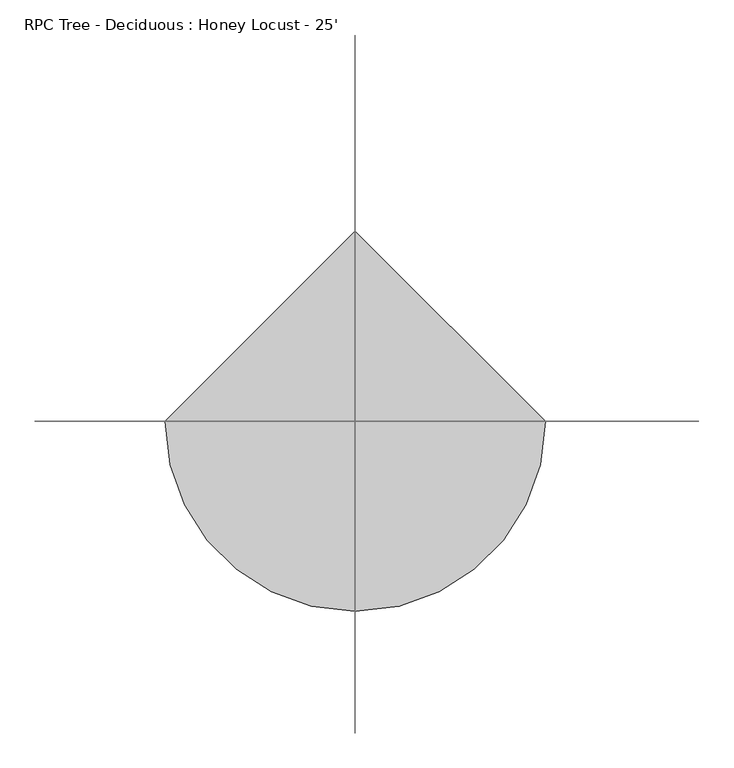
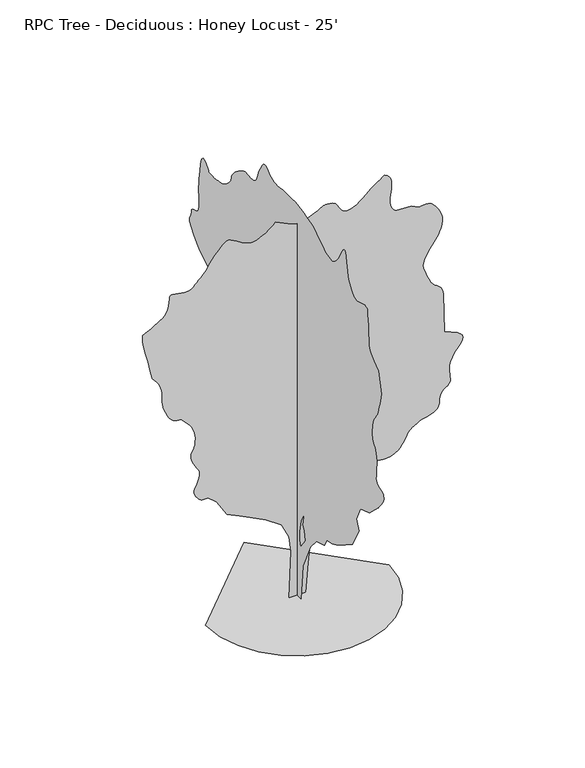
"""IFC4 building model written with IfcOpenShell, lengths in millimetres: geographic element geometry, RPC Tree - Deciduous : Honey Locust - 25'."""

from ifc_helpers import new_model, si_unit, origin, place, context, project, spatial, triangles, source, transform, mapped, element, save


def rpc_tree_deciduous_honey_locust_25_cc46a1f1(model_context):
    return source(origin(), model_context, "Body", "Tessellation", [
        triangles([(0.0017564, 138.2462219, 0.0), (0.0017564, -127.0105432, 0.0), (0.0017564, -184.6753374, 668.9082985), (0.0017564, -426.8668951, 1176.3566122), (0.0017564, -611.3926231, 1395.4822632), (0.0017564, -865.1155083, 1476.2135273), (0.0017564, -934.3152088, 1614.6078415), (0.0017564, -1118.8409369, 1660.7391827), (0.0017564, -1168.1321142, 1679.0297813), (0.0017564, -1234.9772346, 1712.4509972), (0.0017564, -1316.4476978, 1758.4833618), (0.0017564, -1409.6173016, 1814.6021748), (0.0017564, -1511.5651485, 1878.2849155), (0.0017564, -1619.3626385, 1947.0122612), (0.0017564, -1730.0862579, 2018.2590752), (0.0017564, -1937.6776566, 2398.8447109), (0.0017564, -1856.9463924, 2583.3806854), (0.0017564, -1983.8091431, 2848.632518), (0.0017564, -2272.1318058, 2952.4168808), (0.0017564, -2537.389016, 3206.1371498), (0.0017564, -2543.9089668, 3214.0110878), (0.0017564, -2561.3334846, 3235.1946785), (0.0017564, -2586.4031754, 3266.0558762), (0.0017564, -2615.9435234, 3302.9873428), (0.0017564, -2646.6774033, 3342.3317436), (0.0017564, -2675.3794304, 3380.4573235), (0.0017564, -2698.8489281, 3413.7311646), (0.0017564, -2714.4444878, 3444.5414932), (0.0017564, -2721.9882133, 3476.5453537), (0.0017564, -2721.8358971, 3508.1684235), (0.0017564, -2714.4444878, 3537.73377), (0.0017564, -2700.1950668, 3563.6926506), (0.0017564, -2679.4940048, 3584.4190018), (0.0017564, -2652.7226738, 3598.2620522), (0.0017564, -2621.3536583, 3608.345739), (0.0017564, -2588.1556847, 3619.6488281), (0.0017564, -2555.5675575, 3633.3648514), (0.0017564, -2526.024884, 3650.7129204), (0.0017564, -2501.9153091, 3672.9124374), (0.0017564, -2485.67444, 3701.157225), (0.0017564, -2479.7233498, 3736.6663948), (0.0017564, -2481.5749809, 3780.2273987), (0.0017564, -2486.0453476, 3831.0780739), (0.0017564, -2491.5266991, 3887.9740196), (0.0017564, -2496.4008202, 3949.6961243), (0.0017564, -2499.0579254, 4015.0755638), (0.0017564, -2497.8818344, 4082.8426483), (0.0017564, -2491.2575294, 4151.8544243), (0.0017564, -2477.5720276, 4213.7541344), (0.0017564, -2458.0368828, 4262.9284584), (0.0017564, -2435.2733013, 4302.24757), (0.0017564, -2411.9053963, 4334.4801956), (0.0017564, -2390.5542286, 4362.4965088), (0.0017564, -2373.8434753, 4389.0902344), (0.0017564, -2364.3947788, 4417.1062569), (0.0017564, -2359.5864967, 4450.1263344), (0.0017564, -2355.5860142, 4489.1913918), (0.0017564, -2353.1983692, 4533.3113731), (0.0017564, -2353.2315067, 4581.4694801), (0.0017564, -2356.4927902, 4632.6250786), (0.0017564, -2363.7901646, 4685.8128204), (0.0017564, -2375.9288132, 4740.016198), (0.0017564, -2392.0679443, 4787.9461212), (0.0017564, -2410.4271435, 4825.3601166), (0.0017564, -2430.3991802, 4855.916391), (0.0017564, -2451.3794403, 4883.2722794), (0.0017564, -2472.7636002, 4911.0089584), (0.0017564, -2493.9471909, 4942.7843445), (0.0017564, -2514.3232727, 4982.2051941), (0.0017564, -2534.0944496, 5031.4045166), (0.0017564, -2553.8659172, 5089.0626251), (0.0017564, -2573.6269203, 5153.8075104), (0.0017564, -2593.4135033, 5224.1654251), (0.0017564, -2613.1747971, 5298.7905212), (0.0017564, -2632.9360909, 5376.2096329), (0.0017564, -2652.7226738, 5455.0763306), (0.0017564, -2548.9127312, 5835.6443802), (0.0017564, -2410.52612, 5939.4537415), (0.0017564, -2376.165136, 5966.8602081), (0.0017564, -2343.2136589, 5995.5625259), (0.0017564, -2313.0867188, 6026.9059616), (0.0017564, -2287.1965839, 6062.1863663), (0.0017564, -2266.9553776, 6102.6995911), (0.0017564, -2253.772752, 6149.7659042), (0.0017564, -2249.0662079, 6204.705574), (0.0017564, -2247.7225399, 6269.3992996), (0.0017564, -2243.9556187, 6343.7709229), (0.0017564, -2238.1721054, 6426.2187973), (0.0017564, -2230.7756092, 6515.1186035), (0.0017564, -2222.1675591, 6608.8704391), (0.0017564, -2212.7518547, 6705.8220795), (0.0017564, -2202.9347214, 6804.4247818), (0.0017564, -2185.5179066, 6814.1270966), (0.0017564, -2167.3950302, 6822.8393555), (0.0017564, -2147.8598854, 6829.5453415), (0.0017564, -2126.2064106, 6833.2026764), (0.0017564, -2101.7285442, 6832.8218857), (0.0017564, -2073.7199341, 6827.4117508), (0.0017564, -2041.4746639, 6815.9560547), (0.0017564, -2006.8748863, 6801.3255524), (0.0017564, -1972.2775795, 6787.914743), (0.0017564, -1937.6776566, 6776.9165771), (0.0017564, -1903.077879, 6769.5501663), (0.0017564, -1868.4805721, 6767.0357849), (0.0017564, -1833.8806492, 6770.5663834), (0.0017564, -1799.2833424, 6781.3616547), (0.0017564, -1765.6919334, 6801.5546082), (0.0017564, -1733.9191635, 6831.4504578), (0.0017564, -1703.6576385, 6869.42314), (0.0017564, -1674.6050514, 6913.8221741), (0.0017564, -1646.4618565, 6963.0982361), (0.0017564, -1618.9257465, 7015.5746841), (0.0017564, -1591.689473, 7069.6766144), (0.0017564, -1522.4922432, 7484.8646439), (0.0017564, -1510.0182953, 7494.262326), (0.0017564, -1496.8382858, 7500.8665741), (0.0017564, -1482.2460079, 7501.8060516), (0.0017564, -1465.5354, 7494.262326), (0.0017564, -1446.0002552, 7475.4413818), (0.0017564, -1422.9345119, 7442.4974625), (0.0017564, -1395.6321087, 7392.5865555), (0.0017564, -1366.480545, 7335.9952423), (0.0017564, -1337.5296959, 7284.4588531), (0.0017564, -1307.5703327, 7237.3669601), (0.0017564, -1275.393663, 7194.085881), (0.0017564, -1239.7855167, 7154.0296051), (0.0017564, -1199.5366653, 7116.6156097), (0.0017564, -1153.4407871, 7081.2078873), (0.0017564, -1100.9873028, 7057.7133911), (0.0017564, -1043.0880753, 7054.1827927), (0.0017564, -980.6472645, 7067.2889694), (0.0017564, -914.5768787, 7093.7047989), (0.0017564, -845.7836214, 7130.1287384), (0.0017564, -775.1741959, 7173.2069229), (0.0017564, -703.6555235, 7219.6128113), (0.0017564, -659.2741482, 7251.5405136), (0.0017564, -615.4946983, 7282.3758408), (0.0017564, -572.9269114, 7311.0014191), (0.0017564, -532.1751838, 7336.2748764), (0.0017564, -493.8440932, 7357.1282547), (0.0017564, -458.5406522, 7372.4186005), (0.0017564, -426.8668951, 7381.0547012), (0.0017564, -379.7931333, 7391.6464966), (0.0017564, -304.4771091, 7410.7220764), (0.0017564, -210.8004869, 7434.013678), (0.0017564, -108.6519436, 7457.3308594), (0.0017564, -7.915369, 7476.3808594), (0.0017564, 81.5235032, 7486.9726547), (0.0017564, 149.779584, 7484.8646439), (0.0017564, 204.0816928, 7478.1336594), (0.0017564, 257.9799291, 7476.2541229), (0.0017564, 311.0709472, 7476.9907059), (0.0017564, 362.9529548, 7478.1336594), (0.0017564, 413.2194723, 7477.4732346), (0.0017564, 461.4692888, 7472.7485229), (0.0017564, 507.2984682, 7461.8015167), (0.0017564, 555.4821914, 7451.6666702), (0.0017564, 608.9110522, 7450.0156082), (0.0017564, 664.3541433, 7455.4513229), (0.0017564, 718.5906584, 7466.5000671), (0.0017564, 768.3873281, 7481.7909943), (0.0017564, 810.5182594, 7499.9265152), (0.0017564, 841.7526175, 7519.4590439), (0.0017564, 869.6950979, 7543.2081757), (0.0017564, 902.8827524, 7570.9704346), (0.0017564, 939.4967966, 7596.9293152), (0.0017564, 977.728838, 7615.2171524), (0.0017564, 1015.7551506, 7619.9924423), (0.0017564, 1051.7671967, 7605.3875198), (0.0017564, 1083.943939, 7565.5858795), (0.0017564, 1111.584185, 7516.9952408), (0.0017564, 1135.5896965, 7477.701709), (0.0017564, 1156.5725727, 7444.2496811), (0.0017564, 1175.132341, 7413.2114594), (0.0017564, 1191.8760138, 7381.1564392), (0.0017564, 1207.410676, 7344.6819214), (0.0017564, 1222.3407967, 7300.3334656), (0.0017564, 1236.6967518, 7254.9693741), (0.0017564, 1251.0554684, 7217.07285), (0.0017564, 1266.8236919, 7185.6526749), (0.0017564, 1285.4164524, 7159.6432159), (0.0017564, 1308.248489, 7138.103833), (0.0017564, 1336.7269833, 7119.9683121), (0.0017564, 1372.2666744, 7104.2710144), (0.0017564, 1413.6914715, 7095.1529663), (0.0017564, 1457.9408054, 7094.9239105), (0.0017564, 1503.6022625, 7099.7247803), (0.0017564, 1549.2612488, 7105.7447617), (0.0017564, 1593.5105827, 7109.1480423), (0.0017564, 1634.9353798, 7106.0999725), (0.0017564, 1672.1235168, 7092.7397415), (0.0017564, 1714.3205051, 7068.3051865), (0.0017564, 1768.2192501, 7035.5897415), (0.0017564, 1828.5747231, 6996.1944717), (0.0017564, 1890.1391338, 6951.7954376), (0.0017564, 1947.6700699, 6903.9419632), (0.0017564, 1995.9198864, 6854.2845291), (0.0017564, 2029.6434093, 6804.4247818), (0.0017564, 2047.5985634, 6762.5657089), (0.0017564, 2056.0720287, 6732.1873306), (0.0017564, 2061.1140175, 6707.879512), (0.0017564, 2068.7821541, 6684.1809586), (0.0017564, 2085.1219997, 6655.6315384), (0.0017564, 2116.1913242, 6616.7949554), (0.0017564, 2168.0377235, 6562.2360764), (0.0017564, 2230.1762272, 6507.9306702), (0.0017564, 2288.0754547, 6470.9736237), (0.0017564, 2341.7380222, 6447.5297058), (0.0017564, 2391.1637844, 6433.7881027), (0.0017564, 2436.3553574, 6425.8885849), (0.0017564, 2477.3077995, 6419.9959213), (0.0017564, 2514.0259071, 6412.2998795), (0.0017564, 2553.510125, 6405.0352066), (0.0017564, 2599.6366699, 6402.2161926), (0.0017564, 2647.7694878, 6402.6225632), (0.0017564, 2693.3117661, 6405.0352066), (0.0017564, 2731.5640823, 6408.2611725), (0.0017564, 2757.9293335, 6411.0807678), (0.0017564, 2767.7589661, 6412.2998795), (0.0017564, 2779.3922676, 6430.4609802), (0.0017564, 2809.9738312, 6472.8281616), (0.0017564, 2853.0775955, 6521.2403229), (0.0017564, 2902.2519196, 6557.5625244), (0.0017564, 2950.9945839, 6563.6075043), (0.0017564, 2992.9045258, 6521.2403229), (0.0017564, 3021.4792351, 6412.2998795), (0.0017564, 3039.1830963, 6281.2613663), (0.0017564, 3053.0770157, 6180.2965988), (0.0017564, 3063.5417839, 6102.7251709), (0.0017564, 3070.9584824, 6041.8916748), (0.0017564, 3075.7846413, 5991.1680267), (0.0017564, 3078.3751808, 5943.8482407), (0.0017564, 3079.1373436, 5893.3274872), (0.0017564, 3077.918232, 5838.9459229), (0.0017564, 3075.0986366, 5784.5899384), (0.0017564, 3071.8729614, 5730.2089554), (0.0017564, 3069.4600273, 5675.8273911), (0.0017564, 3069.0536568, 5621.4714066), (0.0017564, 3071.8729614, 5567.0904236), (0.0017564, 3079.1373436, 5512.7344391), (0.0017564, 3099.1779808, 5469.782991), (0.0017564, 3134.966494, 5444.6112717), (0.0017564, 3179.5942932, 5429.5238205), (0.0017564, 3226.2792343, 5416.8495941), (0.0017564, 3268.113018, 5398.9169678), (0.0017564, 3298.2376328, 5368.0816406), (0.0017564, 3309.7944855, 5316.6719879), (0.0017564, 3318.6843498, 5264.1193817), (0.0017564, 3338.4456436, 5228.1023941), (0.0017564, 3358.8164932, 5198.3588608), (0.0017564, 3369.5097359, 5164.551622), (0.0017564, 3360.2387901, 5116.4440933), (0.0017564, 3320.6912041, 5043.7235321), (0.0017564, 3240.6051041, 4936.0789398), (0.0017564, 3137.9128258, 4824.090136), (0.0017564, 3039.0560692, 4740.5243065), (0.0017564, 2946.4477684, 4678.5737274), (0.0017564, 2862.5264374, 4631.3298088), (0.0017564, 2789.7047195, 4591.9598282), (0.0017564, 2730.395549, 4553.5804848), (0.0017564, 2687.0124413, 4509.3590561), (0.0017564, 2658.1580978, 4464.7821259), (0.0017564, 2638.3970947, 4426.6568367), (0.0017564, 2624.0715157, 4390.1317406), (0.0017564, 2611.574604, 4350.4059677), (0.0017564, 2597.249025, 4302.5777824), (0.0017564, 2577.462442, 4241.8466057), (0.0017564, 2548.6333878, 4163.3859879), (0.0017564, 2517.7242279, 4078.1182274), (0.0017564, 2493.4823936, 3999.5052933), (0.0017564, 2474.7855698, 3926.4298119), (0.0017564, 2460.5312073, 3857.7988266), (0.0017564, 2449.6039673, 3792.521125), (0.0017564, 2440.8943245, 3729.4275925), (0.0017564, 2433.294643, 3667.4770134), (0.0017564, 2455.3521629, 3642.6102173), (0.0017564, 2476.2994308, 3616.9562599), (0.0017564, 2495.0267761, 3589.7021095), (0.0017564, 2510.4267082, 3560.0097359), (0.0017564, 2521.3894112, 3527.0913963), (0.0017564, 2526.8021622, 3490.1343498), (0.0017564, 2525.5600868, 3448.3514351), (0.0017564, 2526.3652702, 3406.9748909), (0.0017564, 2533.4264671, 3370.2718987), (0.0017564, 2538.8723557, 3335.7786552), (0.0017564, 2534.8385902, 3301.0569374), (0.0017564, 2513.4544304, 3263.7443893), (0.0017564, 2466.850589, 3221.3772079), (0.0017564, 2387.1633018, 3171.5424591), (0.0017564, 2299.4063038, 3131.0039452), (0.0017564, 2230.2092194, 3111.2173622), (0.0017564, 2174.1235439, 3101.9464165), (0.0017564, 2125.7061504, 3092.878656), (0.0017564, 2079.5060635, 3073.7016289), (0.0017564, 2030.0803013, 3034.1540428), (0.0017564, 1971.9778885, 2963.9484444), (0.0017564, 1918.922406, 2886.046804), (0.0017564, 1885.02869, 2826.5091591), (0.0017564, 1865.4579369, 2779.671611), (0.0017564, 1855.3716339, 2739.8952599), (0.0017564, 1849.9258907, 2701.5159164), (0.0017564, 1844.2769623, 2658.9202606), (0.0017564, 1833.5835743, 2606.4438126), (0.0017564, 1823.3625412, 2556.2026932), (0.0017564, 1818.1834969, 2520.8993248), (0.0017564, 1811.7953693, 2495.6822594), (0.0017564, 1797.9422905, 2475.7102226), (0.0017564, 1770.3705723, 2456.1393242), (0.0017564, 1722.8269627, 2432.1339581), (0.0017564, 1649.0577736, 2398.8447109), (0.0017564, 1567.2851486, 2366.9372108), (0.0017564, 1497.6180347, 2346.9297112), (0.0017564, 1436.6226299, 2333.7851646), (0.0017564, 1380.8747246, 2322.4516994), (0.0017564, 1326.9429874, 2307.8950298), (0.0017564, 1271.3957966, 2285.0629932), (0.0017564, 1210.806617, 2248.9188332), (0.0017564, 1144.870816, 2202.0812851), (0.0017564, 1075.9099091, 2151.0044609), (0.0017564, 1004.4242289, 2096.4021252), (0.0017564, 930.9242821, 2038.9727818), (0.0017564, 855.9105469, 1979.4251083), (0.0017564, 779.8858995, 1918.4651665), (0.0017564, 703.3583033, 1856.7991631), (0.0017564, 276.64129, 1533.8765774), (0.0017564, 149.779584, 1314.7509991), (0.0017564, 115.1805058, 1141.7593054), (0.0017564, 103.6476433, 876.5023132), (0.0020752, -103.9448272, 980.2967772), (0.0020752, -80.8791112, 1107.1595278), (0.0020752, -80.8791112, 1268.6195126), (0.0020752, -127.0105432, 1499.2792706), (0.0020752, -230.8067694, 1706.8706692), (0.0020752, -184.6753374, 1453.147784), (0.0020752, -230.8067694, 1372.4165199), (0.0020752, -265.4043305, 1199.4223555), (154.7882082, 0.0004434, 0.0162828), (-145.0671264, 0.0004434, 0.0162828), (-110.4685569, 0.0003925, 876.5175739), (-145.0671264, 0.000378, 1164.8403093), (-283.4611681, 0.0003635, 1441.6288651), (-560.2523217, 0.0003489, 1637.6887001), (-963.9036644, 0.0003344, 1845.2827148), (-1263.7605068, 0.0003271, 1983.677029), (-1459.8203419, 0.0003126, 2295.065435), (-1609.7462196, 0.000298, 2421.9281857), (-1636.8810459, 0.0003053, 2419.6396626), (-1663.7135651, 0.0003053, 2418.4637169), (-1689.9389992, 0.0003053, 2419.5050777), (-1715.2578026, 0.000298, 2423.8764679), (-1739.3649067, 0.000298, 2432.6877033), (-1761.9606205, 0.000298, 2447.0436584), (-1782.7404568, 0.000298, 2468.0595268), (-1802.9155334, 0.000298, 2493.4774521), (-1822.6843849, 0.000298, 2520.3098259), (-1840.2357845, 0.0002908, 2548.5572296), (-1853.7537094, 0.0002908, 2578.199025), (-1861.4193752, 0.0002908, 2609.2886971), (-1861.4193752, 0.0002908, 2641.7497971), (-1851.9375412, 0.0002835, 2675.6587738), (-1833.5784874, 0.0002835, 2714.1904335), (-1810.985099, 0.0002835, 2759.3769196), (-1788.3893852, 0.0002762, 2809.4148537), (-1770.0301861, 0.0002762, 2862.4755684), (-1760.1445976, 0.000269, 2916.7298149), (-1762.9689892, 0.000269, 2970.4000854), (-1782.7404568, 0.000269, 3021.631842), (-1812.8012672, 0.0002617, 3069.7646599), (-1842.4557072, 0.0002617, 3115.6624397), (-1869.8928406, 0.0002544, 3159.9347374), (-1893.2963539, 0.0002544, 3203.2161072), (-1910.8477535, 0.0002544, 3246.0658173), (-1920.7308712, 0.0002471, 3289.1442924), (-1921.134771, 0.0002471, 3333.0355087), (-1913.6366821, 0.0002471, 3370.6526894), (-1902.1049732, 0.0002399, 3398.1864738), (-1888.1503017, 0.0002399, 3421.0972847), (-1873.3903015, 0.0002399, 3444.7952568), (-1859.43563, 0.0002399, 3474.7419754), (-1847.9014503, 0.0002399, 3516.397863), (-1840.4059776, 0.0002326, 3575.2242142), (-1839.1614315, 0.0002253, 3640.3751793), (-1844.5740372, 0.0002253, 3698.2870514), (-1855.534124, 0.0002253, 3750.1283638), (-1870.9342014, 0.0002181, 3797.143808), (-1889.6641628, 0.0002181, 3840.5016266), (-1910.6114307, 0.0002181, 3881.4718002), (-1932.6688053, 0.0002108, 3921.1972824), (-2094.1288628, 0.0002035, 4094.1966064), (-2131.1822697, 0.0002035, 4094.6791351), (-2168.1342293, 0.0002035, 4097.9556793), (-2204.8854744, 0.0002035, 4106.8964127), (-2241.3344124, 0.0002035, 4124.3209305), (-2277.3769798, 0.0001963, 4153.0482468), (-2312.9191418, 0.0001963, 4195.8726677), (-2347.8542187, 0.000189, 4255.6640762), (-2378.9895275, 0.000189, 4321.6024933), (-2403.4675392, 0.0001817, 4382.0799065), (-2421.6893921, 0.0001817, 4438.7470871), (-2434.0643635, 0.0001817, 4493.1792297), (-2440.9908302, 0.0001745, 4547.0018166), (-2442.8729828, 0.0001745, 4601.8403297), (-2440.1170464, 0.0001672, 4659.3205421), (-2439.9138611, 0.0001672, 4717.8166809), (-2448.3874718, 0.0001599, 4774.3062561), (-2464.3234177, 0.0001599, 4828.1797119), (-2486.5177025, 0.0001527, 4878.801622), (-2513.751796, 0.0001527, 4925.6138809), (-2544.8234459, 0.0001527, 4967.9810623), (-2578.5039482, 0.0001454, 5005.2933197), (-2606.1136002, 0.0001454, 5036.2053864), (-2622.8268242, 0.0001454, 5064.6786484), (-2633.2915924, 0.0001454, 5098.2068344), (-2642.1308784, 0.0001381, 5144.2313507), (-2653.9926544, 0.0001381, 5210.2459259), (-2673.5251831, 0.0001308, 5303.6669678), (-2705.3767273, 0.0001236, 5432.0132034), (-2739.5397583, 0.0001163, 5564.8295151), (-2764.0251823, 0.000109, 5669.807991), (-2780.4334831, 0.0001018, 5751.5704422), (-2790.3651443, 0.0001018, 5814.7910019), (-2795.4959358, 9.45e-05, 5864.0920624), (-2797.3754723, 9.45e-05, 5904.0971786), (-2797.6295265, 9.45e-05, 5939.4537415), (-2780.0526924, 9.45e-05, 5947.0736252), (-2760.7486382, 9.45e-05, 5955.7608856), (-2738.0157234, 8.72e-05, 5966.7078918), (-2710.1520172, 8.72e-05, 5980.9576035), (-2675.4047195, 8.72e-05, 5999.6518112), (-2632.0977699, 8.72e-05, 6023.8834717), (-2578.5039482, 8.72e-05, 6054.794957), (-2522.6948547, 8e-05, 6086.4941849), (-2473.739122, 8e-05, 6114.9674469), (-2431.4405411, 8e-05, 6144.0761353), (-2395.5985428, 8e-05, 6177.5787415), (-2366.0102325, 7.27e-05, 6219.387236), (-2342.4746052, 7.27e-05, 6273.2856903), (-2324.7886208, 6.54e-05, 6343.110498), (-2314.1282249, 6.54e-05, 6412.6556717), (-2308.7154739, 5.82e-05, 6464.4205353), (-2303.9071918, 5.82e-05, 6500.4631027), (-2295.0629642, 5.82e-05, 6522.7896469), (-2277.5471729, 5.82e-05, 6533.4320206), (-2246.7141712, 5.82e-05, 6534.3720795), (-2197.9258701, 5.82e-05, 6527.641095), (-2140.092627, 5.82e-05, 6517.4300903), (-2085.4878204, 5.82e-05, 6508.0068283), (-2034.5150597, 5.82e-05, 6501.6060562), (-1987.575919, 5.82e-05, 6500.4631027), (-1945.0767689, 5.82e-05, 6506.7877167), (-1907.4187477, 5.82e-05, 6522.7896469), (-1875.0032845, 5.82e-05, 6550.7042221), (-1844.541045, 5.09e-05, 6583.0894547), (-1812.0595974, 5.09e-05, 6613.4422531), (-1776.9567982, 5.09e-05, 6645.4205338), (-1738.6257076, 5.09e-05, 6682.6572144), (-1696.4617115, 4.36e-05, 6728.7578888), (-1649.8604862, 4.36e-05, 6787.3560562), (-1598.2146561, 3.63e-05, 6862.1078888), (-1546.1980637, 2.91e-05, 6938.7142593), (-1498.4181313, 2.91e-05, 7002.036557), (-1454.1714134, 2.91e-05, 7054.2589508), (-1412.7466164, 2.18e-05, 7097.5911896), (-1373.4401493, 2.18e-05, 7134.268602), (-1335.5459507, 2.18e-05, 7166.5265167), (-1298.3578136, 1.45e-05, 7196.5496841), (-1288.0707962, 1.45e-05, 7208.5129074), (-1275.3606709, 1.45e-05, 7218.1646439), (-1257.8092712, 1.45e-05, 7223.193988), (-1232.9934895, 1.45e-05, 7221.2382935), (-1198.4952318, 1.45e-05, 7210.0116531), (-1151.8939339, 1.45e-05, 7187.1770004), (-1090.7663424, 2.18e-05, 7150.4228485), (-1026.7456861, 2.18e-05, 7109.5544128), (-971.2010387, 2.18e-05, 7076.382019), (-921.3027763, 2.91e-05, 7051.4649353), (-874.2290508, 2.91e-05, 7035.4374252), (-827.1577961, 2.91e-05, 7028.858757), (-777.2595337, 2.91e-05, 7032.3893555), (-721.7123428, 2.91e-05, 7046.6134872), (-664.755427, 2.18e-05, 7068.7365555), (-612.0327003, 2.18e-05, 7095.1018066), (-562.8405722, 2.18e-05, 7124.9976563), (-516.4729082, 2.18e-05, 7157.7131012), (-472.226154, 1.45e-05, 7192.5615555), (-429.3891249, 1.45e-05, 7228.8075989), (-387.2581573, 1.45e-05, 7265.7390656), (-168.1328515, 2.18e-05, 7161.9547028), (-133.3996518, 2.18e-05, 7144.8603973), (-97.8597517, 2.18e-05, 7129.1125214), (-60.7056832, 2.18e-05, 7115.9551849), (-21.1306711, 2.18e-05, 7106.7348175), (21.6722237, 2.18e-05, 7102.77285), (68.5100806, 2.18e-05, 7105.3633896), (120.1896296, 2.18e-05, 7115.8284485), (179.9390167, 2.18e-05, 7135.6656097), (246.5473965, 2.18e-05, 7162.9709198), (314.1646537, 1.45e-05, 7193.9079849), (376.9406911, 1.45e-05, 7224.6165756), (429.0233405, 1.45e-05, 7251.3120392), (464.5629953, 1.45e-05, 7270.1585632), (477.7100126, 1.45e-05, 7277.2703384), (487.5271096, 1.45e-05, 7279.4550888), (513.8897447, 1.45e-05, 7283.4682159), (552.1522711, 1.45e-05, 7285.4494904), (597.6791797, 1.45e-05, 7281.5886795), (645.8273672, 1.45e-05, 7268.0249725), (691.9587811, 1.45e-05, 7240.9737167), (731.4328978, 1.45e-05, 7196.5496841), (761.0238968, 2.18e-05, 7148.2642593), (783.1472557, 2.18e-05, 7111.0787384), (801.640967, 2.18e-05, 7083.3670578), (820.3353928, 2.18e-05, 7063.5298965), (843.065764, 2.91e-05, 7049.9406097), (873.6625883, 2.91e-05, 7040.9998764), (915.9611692, 2.91e-05, 7035.081633), (967.9092339, 2.91e-05, 7039.3999741), (1023.6901314, 2.18e-05, 7059.6435059), (1081.4903097, 2.18e-05, 7091.9775787), (1139.4911299, 2.18e-05, 7132.5925415), (1195.8764963, 1.45e-05, 7177.6520004), (1248.8354004, 1.45e-05, 7223.3207245), (1296.5467323, 1.45e-05, 7265.7390656), (1340.3591743, 7.3e-06, 7303.2803787), (1382.9600624, 7.3e-06, 7337.1637756), (1424.5524364, 7.3e-06, 7368.0246826), (1465.3373016, 7.3e-06, 7396.4723648), (1505.5174072, 0.0, 7423.1172501), (1545.2937584, 0.0, 7448.5168625), (1584.8695404, 0.0, 7473.3327896), (1611.8696365, 0.0, 7460.5568253), (1637.7599167, 0.0, 7445.2658981), (1661.4301289, 0.0, 7424.9206284), (1681.7729279, 7.3e-06, 7397.0060532), (1697.6758816, 7.3e-06, 7359.0327896), (1708.0339703, 7.3e-06, 7308.4108795), (1711.732291, 1.45e-05, 7242.6759384), (1708.6384392, 2.18e-05, 7173.2069229), (1701.1073582, 2.18e-05, 7112.0182159), (1691.7602543, 2.18e-05, 7057.4843353), (1683.2181885, 2.91e-05, 7007.9797989), (1678.1077446, 2.91e-05, 6961.9297028), (1679.0501289, 3.63e-05, 6917.6829849), (1688.6665478, 3.63e-05, 6873.639743), (1703.4950031, 3.63e-05, 6833.8631012), (1718.3209877, 4.36e-05, 6802.5452454), (1733.1494431, 4.36e-05, 6778.3135849), (1747.9780437, 4.36e-05, 6759.7205338), (1762.8064991, 4.36e-05, 6745.3440857), (1777.6324837, 4.36e-05, 6733.8128128), (1792.460939, 4.36e-05, 6723.7035461), (2069.2520382, 4.36e-05, 6712.1716919), (2207.6463524, 5.09e-05, 6642.9823105), (2217.499094, 5.09e-05, 6645.8524841), (2244.0954357, 5.09e-05, 6651.9742035), (2282.9953869, 5.09e-05, 6657.485495), (2329.7669506, 5.09e-05, 6658.5778702), (2379.9675201, 5.09e-05, 6651.3899368), (2429.1595757, 5.09e-05, 6632.0858826), (2472.9034172, 5.09e-05, 6596.8304764), (2512.6797684, 5.82e-05, 6549.0025818), (2551.0463219, 5.82e-05, 6495.1035461), (2585.1840637, 6.54e-05, 6436.1501678), (2612.2350288, 6.54e-05, 6373.1836624), (2629.4307816, 7.27e-05, 6307.1690872), (2633.9011482, 7.27e-05, 6239.1482391), (2622.8268242, 8e-05, 6170.111174), (2602.049604, 8e-05, 6105.620343), (2579.4690056, 8.72e-05, 6049.6132965), (2555.3390831, 8.72e-05, 6000.6680283), (2530.0304535, 8.72e-05, 5957.360788), (2503.8024033, 9.45e-05, 5918.2701508), (2476.9726456, 9.45e-05, 5882.0246887), (2449.837674, 9.45e-05, 5847.2012329), (2408.2121624, 0.0001018, 5785.5299973), (2368.9058407, 0.0001018, 5724.5703461), (2334.2399334, 0.000109, 5665.0327011), (2306.5336304, 0.000109, 5607.603067), (2288.1084469, 0.0001163, 5552.9930283), (2281.2834274, 0.0001163, 5501.9141693), (2288.3777618, 0.0001236, 5455.0763306), (2303.2722015, 0.0001236, 5411.8202499), (2318.5706863, 0.0001236, 5370.1390732), (2334.6768253, 0.0001308, 5328.8892654), (2351.9919022, 0.0001308, 5286.8267166), (2370.922578, 0.0001308, 5242.7578949), (2391.869846, 0.0001381, 5195.4375275), (2415.2378963, 0.0001381, 5143.6982437), (2445.5678764, 0.0001454, 5097.4190918), (2484.1684273, 0.0001454, 5063.0531662), (2526.5989769, 0.0001454, 5034.1479538), (2568.4199707, 0.0001454, 5004.2265244), (2605.2247009, 0.0001527, 4966.8381088), (2632.5041405, 0.0001527, 4915.5301941), (2645.8899513, 0.0001599, 4843.8258499), (2668.9530785, 0.0002035, 4105.72817), (2899.6102203, 0.0002108, 4001.9438072), (2935.957711, 0.0002108, 3979.3123398), (2967.9871513, 0.0002108, 3954.3696762), (2991.3043327, 0.0002108, 3924.7787498), (3001.6420738, 0.0002108, 3888.2280739), (2994.6061661, 0.0002181, 3842.381163), (2965.9041389, 0.0002181, 3784.9518196), (2911.1417839, 0.0002253, 3713.6032677), (2850.7916885, 0.0002326, 3637.2509514), (2806.7987343, 0.0002326, 3565.9279793), (2777.1063606, 0.0002399, 3499.049794), (2759.707132, 0.0002399, 3436.0068398), (2752.6206459, 0.0002471, 3376.1901421), (2753.7891792, 0.0002471, 3319.0145622), (2761.2311668, 0.0002544, 3263.8205475), (2769.4861862, 0.0002544, 3214.1381149), (2773.7280785, 0.0002544, 3172.7107018), (2772.7374413, 0.0002617, 3137.9384056), (2765.2698738, 0.0002617, 3108.2201614), (2750.1315536, 0.0002617, 3081.9313591), (2726.1283676, 0.0002617, 3057.4456444), (2692.0162056, 0.0002617, 3033.1634056), (2656.5834846, 0.000269, 3007.7126335), (2628.8212257, 0.000269, 2980.6616684), (2607.8916893, 0.000269, 2951.756456), (2593.0327126, 0.000269, 2920.8699692), (2583.4315544, 0.0002762, 2887.7484444), (2578.249894, 0.0002762, 2852.2139854), (2576.7002792, 0.0002762, 2814.0378273), (2574.4905304, 0.0002835, 2776.5473831), (2567.4293335, 0.0002835, 2742.8924606), (2554.9071327, 0.0002835, 2712.6663986), (2536.3501259, 0.0002835, 2685.4631172), (2511.1330605, 0.0002908, 2660.9012444), (2478.6539383, 0.0002908, 2638.5238312), (2438.3036396, 0.0002908, 2617.9753761), (2396.3758209, 0.0002908, 2601.9734459), (2358.4816223, 0.0002908, 2591.6357048), (2323.0080608, 0.0002908, 2584.0916885), (2288.3421535, 0.0002908, 2576.5735428), (2252.8710629, 0.0002908, 2566.2102219), (2214.9768642, 0.0002908, 2550.2082916), (2173.0465748, 0.000298, 2525.7225769), (2134.3801849, 0.000298, 2501.648465), (2105.1956291, 0.000298, 2485.6439186), (2082.2644707, 0.000298, 2473.0685234), (2062.3585636, 0.000298, 2459.2838997), (2042.2519421, 0.000298, 2439.6473076), (2018.7163147, 0.0003053, 2409.5203674), (1988.5207741, 0.0003053, 2364.2626648), (1957.3856106, 0.0003053, 2310.7346821), (1930.083062, 0.0003126, 2259.4242966), (1901.9730045, 0.0003126, 2211.1414879), (1868.4170586, 0.0003198, 2166.6889687), (1824.7748096, 0.0003198, 2126.8796253), (1766.4030819, 0.0003198, 2092.5158798), (1688.6665478, 0.0003198, 2064.4058224), (1611.2981598, 0.0003271, 2049.7144226), (1552.6928707, 0.0003271, 2049.9481293), (1506.1906219, 0.0003198, 2057.4462181), (1465.1365871, 0.0003198, 2064.5404072), (1422.8709984, 0.0003198, 2063.5676468), (1372.7390293, 0.0003271, 2046.8544228), (1308.0784412, 0.0003271, 2006.7427723), (1236.0922829, 0.0003271, 1957.583709), (1168.5411009, 0.0003344, 1917.1011509), (1105.630406, 0.0003344, 1882.6715664), (1047.5635288, 0.0003344, 1851.6708424), (994.5385677, 0.0003344, 1821.4753017), (946.7611788, 0.0003416, 1789.4663544), (904.4270622, 0.0003416, 1753.0174164), (863.5407497, 0.0003416, 1713.1393272), (820.2337275, 0.0003489, 1672.6569145), (774.9100405, 0.0003489, 1631.6714802), (727.9708998, 0.0003489, 1590.2796753), (679.8201324, 0.0003562, 1548.5857086), (630.8642544, 0.0003562, 1506.6908821), (581.50702, 0.0003562, 1464.6946083), (339.3157348, 0.000378, 1176.3718729), (235.5192361, 0.0003925, 899.5832445), (200.9196402, 0.0004143, 542.0633883), (-1658.5903313, 0.0, 0.0172132), (-1614.7424263, -380.0394845, 0.0172132), (-1489.866037, -729.0453255, 0.0172132), (-1293.9560474, -1037.0174429, 0.0172132), (-1037.0174429, -1293.9560474, 0.0172132), (-729.0453255, -1489.866037, 0.0172132), (-380.0394845, -1614.7424263, 0.0172132), (7.25e-05, -1658.5903313, 0.0172132), (380.0394845, -1614.7424263, 0.0172132), (729.0453255, -1489.866037, 0.0172132), (1037.0174429, -1293.9560474, 0.0172132), (1293.9560474, -1037.0174429, 0.0172132), (1489.866037, -729.0453255, 0.0172132), (1614.7424263, -380.0394845, 0.0172132), (1658.5903313, 0.0001454, 0.0172132), (-0.0002175, 1658.5903313, 0.0172132)], [[328, 1, 329], [327, 328, 329], [327, 329, 330], [329, 1, 2], [329, 2, 3], [329, 3, 4], [336, 329, 4], [327, 330, 331], [326, 327, 331], [326, 331, 332], [325, 326, 332], [335, 336, 4], [335, 4, 5], [325, 332, 333], [334, 335, 5], [333, 334, 5], [333, 5, 6], [333, 6, 7], [324, 325, 333], [91, 92, 93], [223, 224, 225], [222, 223, 225], [222, 225, 226], [221, 222, 226], [220, 221, 226], [220, 226, 227], [219, 220, 227], [219, 227, 228], [15, 16, 17], [91, 93, 94], [91, 94, 95], [91, 95, 96], [91, 96, 97], [91, 97, 98], [91, 98, 99], [91, 99, 100], [90, 91, 100], [90, 100, 101], [90, 101, 102], [89, 90, 102], [89, 102, 103], [88, 89, 103], [88, 103, 104], [218, 219, 228], [14, 15, 17], [218, 228, 229], [217, 218, 229], [216, 217, 229], [216, 229, 230], [215, 216, 230], [215, 230, 231], [214, 215, 231], [214, 231, 232], [214, 232, 233], [214, 233, 234], [213, 214, 234], [213, 234, 235], [113, 114, 115], [113, 115, 116], [113, 116, 117], [113, 117, 118], [113, 118, 119], [113, 119, 120], [113, 120, 121], [113, 121, 122], [113, 122, 123], [113, 123, 124], [113, 124, 125], [113, 125, 126], [113, 126, 127], [112, 113, 127], [112, 127, 128], [111, 112, 128], [110, 111, 128], [213, 235, 236], [87, 88, 104], [87, 104, 105], [212, 213, 236], [110, 128, 129], [109, 110, 129], [212, 236, 237], [211, 212, 237], [210, 211, 237], [86, 87, 105], [210, 237, 238], [209, 210, 238], [85, 86, 105], [76, 77, 78], [75, 76, 78], [13, 14, 17], [209, 238, 239], [85, 105, 106], [208, 209, 239], [74, 75, 78], [108, 109, 129], [74, 78, 79], [73, 74, 79], [84, 85, 106], [73, 79, 80], [72, 73, 80], [71, 72, 80], [208, 239, 240], [70, 71, 80], [69, 70, 80], [68, 69, 80], [67, 68, 80], [66, 67, 80], [65, 66, 80], [65, 80, 81], [64, 65, 81], [12, 13, 17], [245, 246, 247], [244, 245, 247], [243, 244, 247], [243, 247, 248], [64, 81, 82], [63, 64, 82], [242, 243, 248], [323, 324, 333], [167, 168, 169], [167, 169, 170], [166, 167, 170], [166, 170, 171], [165, 166, 171], [164, 165, 171], [164, 171, 172], [163, 164, 172], [163, 172, 173], [163, 173, 174], [162, 163, 174], [162, 174, 175], [162, 175, 176], [162, 176, 177], [161, 162, 177], [161, 177, 178], [161, 178, 179], [160, 161, 179], [160, 179, 180], [159, 160, 180], [159, 180, 181], [158, 159, 181], [11, 12, 17], [250, 251, 252], [249, 250, 252], [249, 252, 253], [248, 249, 253], [242, 248, 253], [242, 253, 254], [242, 254, 255], [241, 242, 255], [241, 255, 256], [241, 256, 257], [241, 257, 258], [241, 258, 259], [240, 241, 259], [208, 240, 259], [208, 259, 260], [208, 260, 261], [207, 208, 261], [206, 207, 261], [206, 261, 262], [206, 262, 263], [205, 206, 263], [205, 263, 264], [204, 205, 264], [204, 264, 265], [204, 265, 266], [204, 266, 267], [204, 267, 268], [204, 268, 269], [203, 204, 269], [10, 11, 17], [9, 10, 17], [8, 9, 17], [7, 8, 17], [333, 7, 17], [323, 333, 17], [322, 323, 17], [322, 17, 18], [321, 322, 18], [320, 321, 18], [319, 320, 18], [318, 319, 18], [317, 318, 18], [316, 317, 18], [315, 316, 18], [203, 269, 270], [314, 315, 18], [18, 19, 20], [314, 18, 20], [314, 20, 21], [314, 21, 22], [314, 22, 23], [314, 23, 24], [314, 24, 25], [314, 25, 26], [314, 26, 27], [314, 27, 28], [314, 28, 29], [314, 29, 30], [314, 30, 31], [314, 31, 32], [314, 32, 33], [314, 33, 34], [314, 34, 35], [314, 35, 36], [314, 36, 37], [314, 37, 38], [314, 38, 39], [314, 39, 40], [314, 40, 41], [314, 41, 42], [314, 42, 43], [314, 43, 44], [314, 44, 45], [314, 45, 46], [314, 46, 47], [314, 47, 48], [314, 48, 49], [314, 49, 50], [314, 50, 51], [314, 51, 52], [314, 52, 53], [314, 53, 54], [314, 54, 55], [314, 55, 56], [314, 56, 57], [314, 57, 58], [314, 58, 59], [314, 59, 60], [314, 60, 61], [314, 61, 62], [313, 314, 62], [312, 313, 62], [311, 312, 62], [310, 311, 62], [309, 310, 62], [308, 309, 62], [307, 308, 62], [306, 307, 62], [305, 306, 62], [304, 305, 62], [303, 304, 62], [302, 303, 62], [301, 302, 62], [300, 301, 62], [299, 300, 62], [298, 299, 62], [297, 298, 62], [296, 297, 62], [295, 296, 62], [294, 295, 62], [294, 62, 63], [294, 63, 82], [294, 82, 83], [294, 83, 84], [294, 84, 106], [294, 106, 107], [294, 107, 108], [294, 108, 129], [294, 129, 130], [294, 130, 131], [294, 131, 132], [294, 132, 133], [294, 133, 134], [294, 134, 135], [294, 135, 136], [294, 136, 137], [294, 137, 138], [294, 138, 139], [294, 139, 140], [294, 140, 141], [294, 141, 142], [294, 142, 143], [294, 143, 144], [294, 144, 145], [294, 145, 146], [294, 146, 147], [294, 147, 148], [294, 148, 149], [294, 149, 150], [294, 150, 151], [294, 151, 152], [294, 152, 153], [294, 153, 154], [294, 154, 155], [294, 155, 156], [294, 156, 157], [294, 157, 158], [294, 158, 181], [294, 181, 182], [294, 182, 183], [294, 183, 184], [294, 184, 185], [293, 294, 185], [293, 185, 186], [293, 186, 187], [292, 293, 187], [292, 187, 188], [292, 188, 189], [292, 189, 190], [292, 190, 191], [292, 191, 192], [292, 192, 193], [292, 193, 194], [292, 194, 195], [292, 195, 196], [292, 196, 197], [292, 197, 198], [292, 198, 199], [292, 199, 200], [292, 200, 201], [292, 201, 202], [292, 202, 203], [292, 203, 270], [292, 270, 271], [292, 271, 272], [292, 272, 273], [292, 273, 274], [292, 274, 275], [291, 292, 275], [290, 291, 275], [289, 290, 275], [289, 275, 276], [289, 276, 277], [289, 277, 278], [289, 278, 279], [289, 279, 280], [289, 280, 281], [289, 281, 282], [289, 282, 283], [288, 289, 283], [288, 283, 284], [287, 288, 284], [286, 287, 284], [285, 286, 284], [337, 338, 339], [677, 337, 339], [676, 677, 339], [676, 339, 340], [675, 676, 340], [423, 424, 425], [486, 487, 488], [675, 340, 341], [674, 675, 341], [529, 530, 531], [485, 486, 488], [484, 485, 488], [423, 425, 426], [529, 531, 532], [673, 674, 341], [673, 341, 342], [672, 673, 342], [671, 672, 342], [670, 671, 342], [669, 670, 342], [668, 669, 342], [667, 668, 342], [529, 532, 533], [528, 529, 533], [528, 533, 534], [528, 534, 535], [528, 535, 536], [527, 528, 536], [527, 536, 537], [526, 527, 537], [526, 537, 538], [525, 526, 538], [525, 538, 539], [524, 525, 539], [524, 539, 540], [523, 524, 540], [523, 540, 541], [522, 523, 541], [522, 541, 542], [521, 522, 542], [521, 542, 543], [520, 521, 543], [519, 520, 543], [519, 543, 544], [519, 544, 545], [518, 519, 545], [518, 545, 546], [517, 518, 546], [517, 546, 547], [422, 423, 426], [422, 426, 427], [441, 442, 443], [441, 443, 444], [440, 441, 444], [440, 444, 445], [439, 440, 445], [439, 445, 446], [438, 439, 446], [438, 446, 447], [438, 447, 448], [437, 438, 448], [437, 448, 449], [666, 667, 342], [421, 422, 427], [421, 427, 428], [421, 428, 429], [420, 421, 429], [420, 429, 430], [419, 420, 430], [419, 430, 431], [418, 419, 431], [418, 431, 432], [418, 432, 433], [417, 418, 433], [417, 433, 434], [416, 417, 434], [483, 484, 488], [436, 437, 449], [343, 344, 345], [666, 342, 343], [666, 343, 345], [665, 666, 345], [664, 665, 345], [663, 664, 345], [662, 663, 345], [661, 662, 345], [660, 661, 345], [659, 660, 345], [659, 345, 346], [517, 547, 548], [483, 488, 489], [416, 434, 435], [415, 416, 435], [482, 483, 489], [482, 489, 490], [436, 449, 450], [658, 659, 346], [414, 415, 435], [600, 601, 602], [599, 600, 602], [599, 602, 603], [598, 599, 603], [597, 598, 603], [597, 603, 604], [596, 597, 604], [596, 604, 605], [596, 605, 606], [596, 606, 607], [596, 607, 608], [516, 517, 548], [516, 548, 549], [413, 414, 435], [412, 413, 435], [411, 412, 435], [410, 411, 435], [409, 410, 435], [408, 409, 435], [407, 408, 435], [407, 435, 436], [407, 436, 450], [407, 450, 451], [406, 407, 451], [405, 406, 451], [405, 451, 452], [404, 405, 452], [404, 452, 453], [404, 453, 454], [404, 454, 455], [404, 455, 456], [551, 552, 553], [482, 490, 491], [481, 482, 491], [404, 456, 457], [467, 468, 469], [467, 469, 470], [466, 467, 470], [466, 470, 471], [466, 471, 472], [465, 466, 472], [465, 472, 473], [464, 465, 473], [463, 464, 473], [463, 473, 474], [462, 463, 474], [461, 462, 474], [461, 474, 475], [460, 461, 475], [459, 460, 475], [459, 475, 476], [458, 459, 476], [458, 476, 477], [457, 458, 477], [404, 457, 477], [404, 477, 478], [404, 478, 479], [404, 479, 480], [403, 404, 480], [403, 480, 481], [403, 481, 491], [403, 491, 492], [403, 492, 493], [402, 403, 493], [401, 402, 493], [400, 401, 493], [399, 400, 493], [398, 399, 493], [397, 398, 493], [396, 397, 493], [395, 396, 493], [394, 395, 493], [393, 394, 493], [392, 393, 493], [391, 392, 493], [390, 391, 493], [389, 390, 493], [388, 389, 493], [387, 388, 493], [386, 387, 493], [386, 493, 494], [385, 386, 494], [384, 385, 494], [384, 494, 495], [383, 384, 495], [383, 495, 496], [383, 496, 497], [382, 383, 497], [382, 497, 498], [382, 498, 499], [382, 499, 500], [381, 382, 500], [381, 500, 501], [381, 501, 502], [381, 502, 503], [381, 503, 504], [381, 504, 505], [381, 505, 506], [381, 506, 507], [381, 507, 508], [381, 508, 509], [381, 509, 510], [381, 510, 511], [381, 511, 512], [381, 512, 513], [381, 513, 514], [381, 514, 515], [381, 515, 516], [381, 516, 549], [381, 549, 550], [381, 550, 551], [381, 551, 553], [380, 381, 553], [379, 380, 553], [378, 379, 553], [378, 553, 554], [378, 554, 555], [378, 555, 556], [378, 556, 557], [378, 557, 558], [378, 558, 559], [378, 559, 560], [378, 560, 561], [378, 561, 562], [378, 562, 563], [378, 563, 564], [378, 564, 565], [378, 565, 566], [378, 566, 567], [378, 567, 568], [378, 568, 569], [378, 569, 570], [378, 570, 571], [378, 571, 572], [378, 572, 573], [378, 573, 574], [378, 574, 575], [378, 575, 576], [378, 576, 577], [378, 577, 578], [378, 578, 579], [378, 579, 580], [378, 580, 581], [378, 581, 582], [378, 582, 583], [378, 583, 584], [378, 584, 585], [378, 585, 586], [378, 586, 587], [378, 587, 588], [378, 588, 589], [378, 589, 590], [378, 590, 591], [378, 591, 592], [378, 592, 593], [378, 593, 594], [378, 594, 595], [378, 595, 596], [378, 596, 608], [378, 608, 609], [378, 609, 610], [378, 610, 611], [378, 611, 612], [378, 612, 613], [378, 613, 614], [378, 614, 615], [378, 615, 616], [378, 616, 617], [378, 617, 618], [378, 618, 619], [378, 619, 620], [378, 620, 621], [378, 621, 622], [378, 622, 623], [378, 623, 624], [378, 624, 625], [378, 625, 626], [378, 626, 627], [378, 627, 628], [378, 628, 629], [378, 629, 630], [378, 630, 631], [378, 631, 632], [378, 632, 633], [378, 633, 634], [378, 634, 635], [378, 635, 636], [378, 636, 637], [378, 637, 638], [378, 638, 639], [378, 639, 640], [378, 640, 641], [378, 641, 642], [378, 642, 643], [378, 643, 644], [378, 644, 645], [378, 645, 646], [378, 646, 647], [378, 647, 648], [378, 648, 649], [378, 649, 650], [378, 650, 651], [378, 651, 652], [378, 652, 653], [378, 653, 654], [378, 654, 655], [378, 655, 656], [378, 656, 657], [378, 657, 658], [378, 658, 346], [377, 378, 346], [358, 359, 360], [357, 358, 360], [356, 357, 360], [356, 360, 361], [355, 356, 361], [354, 355, 361], [354, 361, 362], [353, 354, 362], [352, 353, 362], [351, 352, 362], [350, 351, 362], [349, 350, 362], [348, 349, 362], [347, 348, 362], [346, 347, 362], [346, 362, 363], [346, 363, 364], [346, 364, 365], [346, 365, 366], [377, 346, 366], [377, 366, 367], [377, 367, 368], [377, 368, 369], [377, 369, 370], [377, 370, 371], [377, 371, 372], [377, 372, 373], [377, 373, 374], [377, 374, 375], [377, 375, 376], [692, 693, 678], [691, 692, 678], [691, 678, 679], [690, 691, 679], [690, 679, 680], [690, 680, 681], [689, 690, 681], [688, 689, 681], [688, 681, 682], [688, 682, 683], [688, 683, 684], [688, 684, 685], [688, 685, 686], [688, 686, 687]], closed=False),
    ])


if __name__ == "__main__":
    model = new_model("IFC4")
    model_context = context("Model", 3, world=origin())
    ifc_project = project(units=[si_unit("LENGTHUNIT", "METRE", prefix="MILLI")], contexts=[model_context])
    site = spatial("IfcSite", under=ifc_project)
    building = spatial("IfcBuilding", under=site)
    placement = place(None, origin())
    rpc_tree_deciduous_honey_locust_25_shape = rpc_tree_deciduous_honey_locust_25_cc46a1f1(model_context)
    element("IfcGeographicElement", 1, ObjectType="RPC Tree - Deciduous : Honey Locust - 25'", at=placement, inside=building, context=model_context, shape_type="MappedRepresentation", body=[
        mapped(rpc_tree_deciduous_honey_locust_25_shape, transform((0.0, 0.0, 0.0), x_axis=(1.0, 0.0, 0.0), y_axis=(0.0, 1.0, 0.0), z_axis=(0.0, 0.0, 1.0))),
    ])
    save(model, "model.ifc")

# Revit data of these elements
# Type "RPC Tree - Deciduous : Honey Locust - 25'"
#   built-in parameter 1005198 = "{2, 15},{39, RPC-16-G2VH-N100-5X50-0000-ST1L-LVER-AU},{1, 0},{1, 0},{2, 13},{1, 8},{5, Color},{1, 0},{1, 0},{3, 0.8},{3, 0.8},{3, 0.8},{1, 8},{7, BBoxMin},{1, 0},{1, 0},{1, 0},{1, 0},{1, 0},{1, 8},{7, BBoxMax},{1, 0},{1, 0},{1, 0},{1, 0},{1, 0},{2, 11},{9, RPCTypeId},{1, 0},{1, 0},{39, RPC-16-G2VH-N100-5X50-0000-ST1L-LVER-AU},{1, 6},{14, RPCPlantHeight},{1, 0},{1, 0},{2, 25},{2, 11},{7, keyword},{1, 0},{1, 0},{34, :RPCs:Trees [General]:Geometry:RPC},{2, 11},{8, category},{1, 0},{1, 0},{15, Trees [General]},{2, 11},{12, LocalizedUID},{1, 0},{1, 0},{12, Honey-Locust},{2, 14},{6, Height},{1, 0},{1, 0},{2, 25},{1, 2},{16, Cast Reflections},{1, 0},{1, 0},{1, 0},{1, 2},{12, Cast Shadows},{1, 0},{1, 0},{1, 1},{1, 2},{9, Lock View},{1, 0},{1, 0},{1, 0},{1, 4},{5, ViewC},{1, 0},{1, 0},{1, 0},{21, assetlibrary_base.fbx},{1, 5},"
#   built-in parameter 1005195 = "RPC-16-G2VH-N100-5X50-0000-ST1L-LVER-AU"
#   Type Comments = "Honey Locust"
#   Assembly Code = "G2050500"
#   Height = 25' - 0"
#   Default Elevation = 0
